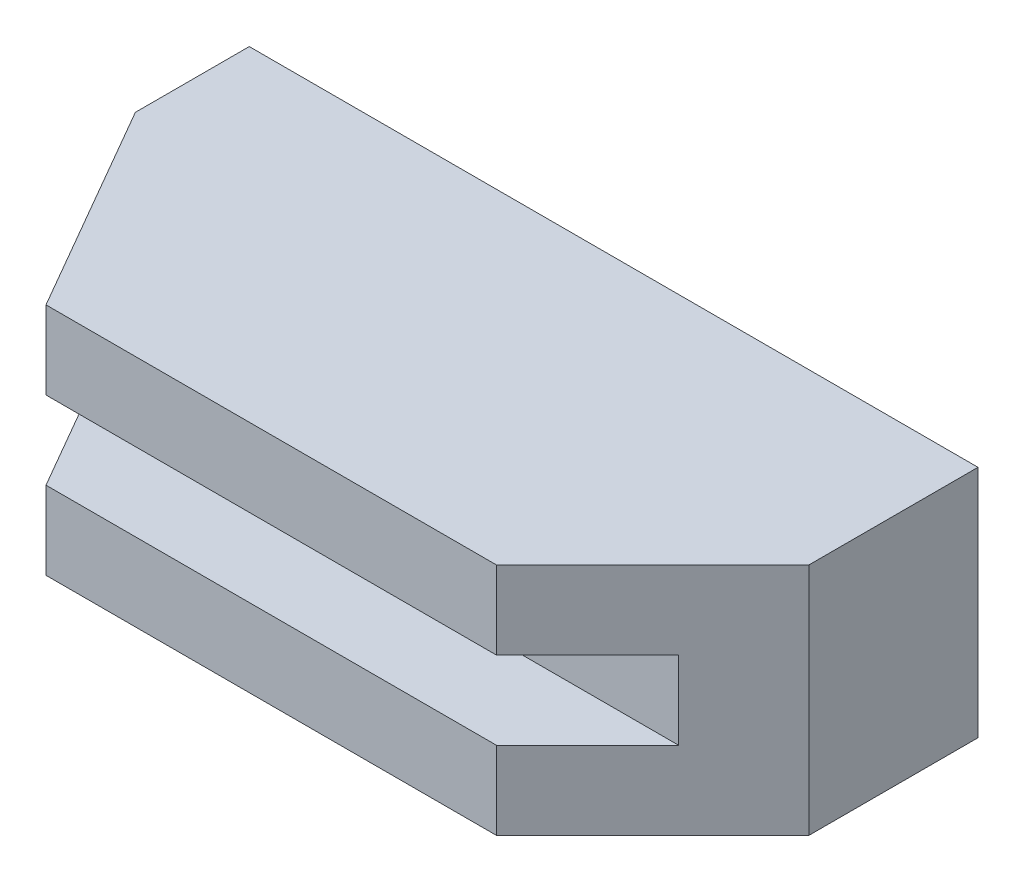
ISO-10303-21;
HEADER;
FILE_DESCRIPTION(('STEP AP214'),'2;1');
FILE_NAME('part.step','',(''),(''),'','','');
FILE_SCHEMA(('AUTOMOTIVE_DESIGN { 1 0 10303 214 1 1 1 1 }'));
ENDSEC;
DATA;
#1=APPLICATION_CONTEXT('core data for automotive mechanical design processes');
#2=APPLICATION_PROTOCOL_DEFINITION('international standard','automotive_design',2000,#1);
#3=PRODUCT_CONTEXT('',#1,'mechanical');
#4=PRODUCT('Part','Part','',(#3));
#5=PRODUCT_RELATED_PRODUCT_CATEGORY('part','',(#4));
#6=PRODUCT_DEFINITION_FORMATION('','',#4);
#7=PRODUCT_DEFINITION_CONTEXT('part definition',#1,'design');
#8=PRODUCT_DEFINITION('design','',#6,#7);
#9=PRODUCT_DEFINITION_SHAPE('','',#8);
#10=(LENGTH_UNIT() NAMED_UNIT(*) SI_UNIT(.MILLI.,.METRE.));
#11=(NAMED_UNIT(*) PLANE_ANGLE_UNIT() SI_UNIT($,.RADIAN.));
#12=(NAMED_UNIT(*) SI_UNIT($,.STERADIAN.) SOLID_ANGLE_UNIT());
#13=UNCERTAINTY_MEASURE_WITH_UNIT(LENGTH_MEASURE(1.E-05),#10,'distance_accuracy_value','');
#14=(GEOMETRIC_REPRESENTATION_CONTEXT(3) GLOBAL_UNCERTAINTY_ASSIGNED_CONTEXT((#13)) GLOBAL_UNIT_ASSIGNED_CONTEXT((#10,
#11,#12)) REPRESENTATION_CONTEXT('',''));
#15=CARTESIAN_POINT('',(0.,0.,0.));
#16=DIRECTION('',(0.,0.,1.));
#17=DIRECTION('',(1.,0.,0.));
#18=AXIS2_PLACEMENT_3D('',#15,#16,#17);
#19=CARTESIAN_POINT('',(0.,0.,25.));
#20=DIRECTION('',(0.,0.,-1.));
#21=DIRECTION('',(-1.,0.,0.));
#22=AXIS2_PLACEMENT_3D('',#19,#20,#21);
#23=PLANE('',#22);
#24=DIRECTION('',(0.,-1.,0.));
#25=VECTOR('',#24,1.);
#26=CARTESIAN_POINT('',(16.0000000000001,9.,25.));
#27=LINE('',#26,#25);
#28=CARTESIAN_POINT('',(16.0000000000001,-3.,25.));
#29=VERTEX_POINT('',#28);
#30=CARTESIAN_POINT('',(16.0000000000001,-9.,25.));
#31=VERTEX_POINT('',#30);
#32=EDGE_CURVE('E142',#29,#31,#27,.T.);
#33=ORIENTED_EDGE('',*,*,#32,.F.);
#34=DIRECTION('',(1.,0.,0.));
#35=VECTOR('',#34,1.);
#36=CARTESIAN_POINT('',(-23.5,-3.,25.));
#37=LINE('',#36,#35);
#38=CARTESIAN_POINT('',(-18.61984811475,-3.,25.));
#39=VERTEX_POINT('',#38);
#40=EDGE_CURVE('E136',#39,#29,#37,.T.);
#41=ORIENTED_EDGE('',*,*,#40,.F.);
#42=DIRECTION('',(0.,-1.,0.));
#43=VECTOR('',#42,1.);
#44=CARTESIAN_POINT('',(-18.61984811475,9.,25.));
#45=LINE('',#44,#43);
#46=CARTESIAN_POINT('',(-18.61984811475,-9.,25.));
#47=VERTEX_POINT('',#46);
#48=EDGE_CURVE('E65',#39,#47,#45,.T.);
#49=ORIENTED_EDGE('',*,*,#48,.T.);
#50=DIRECTION('',(1.,0.,0.));
#51=VECTOR('',#50,1.);
#52=CARTESIAN_POINT('',(-28.,-9.,25.));
#53=LINE('',#52,#51);
#54=EDGE_CURVE('E161',#47,#31,#53,.T.);
#55=ORIENTED_EDGE('',*,*,#54,.T.);
#56=EDGE_LOOP('',(#33,#41,#49,#55));
#57=FACE_BOUND('',#56,.T.);
#58=ADVANCED_FACE('F39',(#57),#23,.F.);
#59=CARTESIAN_POINT('',(28.,-9.,25.));
#60=DIRECTION('',(-1.,0.,0.));
#61=DIRECTION('',(0.,0.,1.));
#62=AXIS2_PLACEMENT_3D('',#59,#60,#61);
#63=PLANE('',#62);
#64=DIRECTION('',(0.,0.,-1.));
#65=VECTOR('',#64,1.);
#66=CARTESIAN_POINT('',(28.,9.,25.));
#67=LINE('',#66,#65);
#68=CARTESIAN_POINT('',(28.,9.,13.));
#69=VERTEX_POINT('',#68);
#70=CARTESIAN_POINT('',(28.,9.,0.));
#71=VERTEX_POINT('',#70);
#72=EDGE_CURVE('E180',#69,#71,#67,.T.);
#73=ORIENTED_EDGE('',*,*,#72,.F.);
#74=DIRECTION('',(0.,-1.,0.));
#75=VECTOR('',#74,1.);
#76=CARTESIAN_POINT('',(28.,9.,13.));
#77=LINE('',#76,#75);
#78=CARTESIAN_POINT('',(28.,-9.,13.));
#79=VERTEX_POINT('',#78);
#80=EDGE_CURVE('E143',#69,#79,#77,.T.);
#81=ORIENTED_EDGE('',*,*,#80,.T.);
#82=DIRECTION('',(0.,0.,-1.));
#83=VECTOR('',#82,1.);
#84=CARTESIAN_POINT('',(28.,-9.,25.));
#85=LINE('',#84,#83);
#86=CARTESIAN_POINT('',(28.,-9.,0.));
#87=VERTEX_POINT('',#86);
#88=EDGE_CURVE('E163',#79,#87,#85,.T.);
#89=ORIENTED_EDGE('',*,*,#88,.T.);
#90=DIRECTION('',(0.,1.,0.));
#91=VECTOR('',#90,1.);
#92=CARTESIAN_POINT('',(28.,-9.,0.));
#93=LINE('',#92,#91);
#94=EDGE_CURVE('E144',#87,#71,#93,.T.);
#95=ORIENTED_EDGE('',*,*,#94,.T.);
#96=EDGE_LOOP('',(#73,#81,#89,#95));
#97=FACE_BOUND('',#96,.T.);
#98=ADVANCED_FACE('F41',(#97),#63,.F.);
#99=CARTESIAN_POINT('',(-28.,9.,25.));
#100=DIRECTION('',(0.,-1.,0.));
#101=DIRECTION('',(0.,0.,-1.));
#102=AXIS2_PLACEMENT_3D('',#99,#100,#101);
#103=PLANE('',#102);
#104=DIRECTION('',(-1.,0.,0.));
#105=VECTOR('',#104,1.);
#106=CARTESIAN_POINT('',(-28.,9.,25.));
#107=LINE('',#106,#105);
#108=CARTESIAN_POINT('',(16.0000000000001,9.,25.));
#109=VERTEX_POINT('',#108);
#110=CARTESIAN_POINT('',(-18.61984811475,9.,25.));
#111=VERTEX_POINT('',#110);
#112=EDGE_CURVE('E157',#109,#111,#107,.T.);
#113=ORIENTED_EDGE('',*,*,#112,.F.);
#114=DIRECTION('',(0.707106781186544,0.,-0.707106781186551));
#115=VECTOR('',#114,1.);
#116=CARTESIAN_POINT('',(28.,9.,13.));
#117=LINE('',#116,#115);
#118=EDGE_CURVE('E140',#109,#69,#117,.T.);
#119=ORIENTED_EDGE('',*,*,#118,.T.);
#120=ORIENTED_EDGE('',*,*,#72,.T.);
#121=DIRECTION('',(-1.,0.,0.));
#122=VECTOR('',#121,1.);
#123=CARTESIAN_POINT('',(-28.,9.,0.));
#124=LINE('',#123,#122);
#125=CARTESIAN_POINT('',(-28.,9.,0.));
#126=VERTEX_POINT('',#125);
#127=EDGE_CURVE('E170',#71,#126,#124,.T.);
#128=ORIENTED_EDGE('',*,*,#127,.T.);
#129=DIRECTION('',(0.,0.,-1.));
#130=VECTOR('',#129,1.);
#131=CARTESIAN_POINT('',(-28.,9.,25.));
#132=LINE('',#131,#130);
#133=CARTESIAN_POINT('',(-28.,9.,8.75310035203402));
#134=VERTEX_POINT('',#133);
#135=EDGE_CURVE('E179',#134,#126,#132,.T.);
#136=ORIENTED_EDGE('',*,*,#135,.F.);
#137=DIRECTION('',(0.500000000000001,0.,0.866025403784438));
#138=VECTOR('',#137,1.);
#139=CARTESIAN_POINT('',(-28.,9.,8.75310035203402));
#140=LINE('',#139,#138);
#141=EDGE_CURVE('E149',#134,#111,#140,.T.);
#142=ORIENTED_EDGE('',*,*,#141,.T.);
#143=EDGE_LOOP('',(#113,#119,#120,#128,#136,#142));
#144=FACE_BOUND('',#143,.T.);
#145=ADVANCED_FACE('F212',(#144),#103,.F.);
#146=CARTESIAN_POINT('',(-28.,-9.,25.));
#147=DIRECTION('',(1.,0.,0.));
#148=DIRECTION('',(0.,0.,-1.));
#149=AXIS2_PLACEMENT_3D('',#146,#147,#148);
#150=PLANE('',#149);
#151=DIRECTION('',(0.,0.,-1.));
#152=VECTOR('',#151,1.);
#153=CARTESIAN_POINT('',(-28.,-9.,25.));
#154=LINE('',#153,#152);
#155=CARTESIAN_POINT('',(-28.,-9.,8.75310035203402));
#156=VERTEX_POINT('',#155);
#157=CARTESIAN_POINT('',(-28.,-9.,0.));
#158=VERTEX_POINT('',#157);
#159=EDGE_CURVE('E176',#156,#158,#154,.T.);
#160=ORIENTED_EDGE('',*,*,#159,.F.);
#161=DIRECTION('',(0.,-1.,0.));
#162=VECTOR('',#161,1.);
#163=CARTESIAN_POINT('',(-28.,9.,8.75310035203402));
#164=LINE('',#163,#162);
#165=EDGE_CURVE('E155',#134,#156,#164,.T.);
#166=ORIENTED_EDGE('',*,*,#165,.F.);
#167=ORIENTED_EDGE('',*,*,#135,.T.);
#168=DIRECTION('',(0.,-1.,0.));
#169=VECTOR('',#168,1.);
#170=CARTESIAN_POINT('',(-28.,-9.,0.));
#171=LINE('',#170,#169);
#172=EDGE_CURVE('E168',#126,#158,#171,.T.);
#173=ORIENTED_EDGE('',*,*,#172,.T.);
#174=EDGE_LOOP('',(#160,#166,#167,#173));
#175=FACE_BOUND('',#174,.T.);
#176=ADVANCED_FACE('F220',(#175),#150,.F.);
#177=CARTESIAN_POINT('',(-28.,-9.,25.));
#178=DIRECTION('',(0.,1.,0.));
#179=DIRECTION('',(0.,0.,1.));
#180=AXIS2_PLACEMENT_3D('',#177,#178,#179);
#181=PLANE('',#180);
#182=ORIENTED_EDGE('',*,*,#88,.F.);
#183=DIRECTION('',(0.707106781186544,0.,-0.707106781186551));
#184=VECTOR('',#183,1.);
#185=CARTESIAN_POINT('',(28.,-9.,13.));
#186=LINE('',#185,#184);
#187=EDGE_CURVE('E160',#31,#79,#186,.T.);
#188=ORIENTED_EDGE('',*,*,#187,.F.);
#189=ORIENTED_EDGE('',*,*,#54,.F.);
#190=DIRECTION('',(0.500000000000001,0.,0.866025403784438));
#191=VECTOR('',#190,1.);
#192=CARTESIAN_POINT('',(-28.,-9.,8.75310035203402));
#193=LINE('',#192,#191);
#194=EDGE_CURVE('E153',#156,#47,#193,.T.);
#195=ORIENTED_EDGE('',*,*,#194,.F.);
#196=ORIENTED_EDGE('',*,*,#159,.T.);
#197=DIRECTION('',(1.,0.,0.));
#198=VECTOR('',#197,1.);
#199=CARTESIAN_POINT('',(-28.,-9.,0.));
#200=LINE('',#199,#198);
#201=EDGE_CURVE('E165',#158,#87,#200,.T.);
#202=ORIENTED_EDGE('',*,*,#201,.T.);
#203=EDGE_LOOP('',(#182,#188,#189,#195,#196,#202));
#204=FACE_BOUND('',#203,.T.);
#205=ADVANCED_FACE('F201',(#204),#181,.F.);
#206=CARTESIAN_POINT('',(-18.61984811475,3.,25.));
#207=VERTEX_POINT('',#206);
#208=EDGE_CURVE('E134',#111,#207,#45,.T.);
#209=ORIENTED_EDGE('',*,*,#208,.T.);
#210=DIRECTION('',(-1.,0.,0.));
#211=VECTOR('',#210,1.);
#212=CARTESIAN_POINT('',(-23.5,3.,25.));
#213=LINE('',#212,#211);
#214=CARTESIAN_POINT('',(16.0000000000001,3.,25.));
#215=VERTEX_POINT('',#214);
#216=EDGE_CURVE('E119',#215,#207,#213,.T.);
#217=ORIENTED_EDGE('',*,*,#216,.F.);
#218=EDGE_CURVE('E132',#109,#215,#27,.T.);
#219=ORIENTED_EDGE('',*,*,#218,.F.);
#220=ORIENTED_EDGE('',*,*,#112,.T.);
#221=EDGE_LOOP('',(#209,#217,#219,#220));
#222=FACE_BOUND('',#221,.T.);
#223=ADVANCED_FACE('F131',(#222),#23,.F.);
#224=CARTESIAN_POINT('',(0.,0.,0.));
#225=DIRECTION('',(0.,0.,-1.));
#226=DIRECTION('',(-1.,0.,0.));
#227=AXIS2_PLACEMENT_3D('',#224,#225,#226);
#228=PLANE('',#227);
#229=ORIENTED_EDGE('',*,*,#94,.F.);
#230=ORIENTED_EDGE('',*,*,#201,.F.);
#231=ORIENTED_EDGE('',*,*,#172,.F.);
#232=ORIENTED_EDGE('',*,*,#127,.F.);
#233=EDGE_LOOP('',(#229,#230,#231,#232));
#234=FACE_BOUND('',#233,.T.);
#235=ADVANCED_FACE('F211',(#234),#228,.T.);
#236=CARTESIAN_POINT('',(-28.,9.,8.75310035203402));
#237=DIRECTION('',(0.866025403784438,0.,-0.500000000000001));
#238=DIRECTION('',(-0.500000000000001,0.,-0.866025403784438));
#239=AXIS2_PLACEMENT_3D('',#236,#237,#238);
#240=PLANE('',#239);
#241=ORIENTED_EDGE('',*,*,#48,.F.);
#242=DIRECTION('',(-0.500000000000001,0.,-0.866025403784438));
#243=VECTOR('',#242,1.);
#244=CARTESIAN_POINT('',(-28.,-3.,8.75310035203402));
#245=LINE('',#244,#243);
#246=CARTESIAN_POINT('',(-22.6612999990774,-3.,18.));
#247=VERTEX_POINT('',#246);
#248=EDGE_CURVE('E154',#39,#247,#245,.T.);
#249=ORIENTED_EDGE('',*,*,#248,.T.);
#250=DIRECTION('',(0.,1.,0.));
#251=VECTOR('',#250,1.);
#252=CARTESIAN_POINT('',(-22.6612999990774,9.,18.));
#253=LINE('',#252,#251);
#254=CARTESIAN_POINT('',(-22.6612999990774,3.,18.));
#255=VERTEX_POINT('',#254);
#256=EDGE_CURVE('E183',#247,#255,#253,.T.);
#257=ORIENTED_EDGE('',*,*,#256,.T.);
#258=DIRECTION('',(0.500000000000001,0.,0.866025403784438));
#259=VECTOR('',#258,1.);
#260=CARTESIAN_POINT('',(-28.,3.,8.75310035203402));
#261=LINE('',#260,#259);
#262=EDGE_CURVE('E189',#255,#207,#261,.T.);
#263=ORIENTED_EDGE('',*,*,#262,.T.);
#264=ORIENTED_EDGE('',*,*,#208,.F.);
#265=ORIENTED_EDGE('',*,*,#141,.F.);
#266=ORIENTED_EDGE('',*,*,#165,.T.);
#267=ORIENTED_EDGE('',*,*,#194,.T.);
#268=EDGE_LOOP('',(#241,#249,#257,#263,#264,#265,#266,#267));
#269=FACE_BOUND('',#268,.T.);
#270=ADVANCED_FACE('F188',(#269),#240,.F.);
#271=CARTESIAN_POINT('',(28.,9.,13.));
#272=DIRECTION('',(-0.707106781186551,0.,-0.707106781186544));
#273=DIRECTION('',(-0.707106781186544,0.,0.707106781186551));
#274=AXIS2_PLACEMENT_3D('',#271,#272,#273);
#275=PLANE('',#274);
#276=DIRECTION('',(0.,-1.,0.));
#277=VECTOR('',#276,1.);
#278=CARTESIAN_POINT('',(23.0000000000001,9.,18.));
#279=LINE('',#278,#277);
#280=CARTESIAN_POINT('',(23.0000000000001,3.,18.));
#281=VERTEX_POINT('',#280);
#282=CARTESIAN_POINT('',(23.0000000000001,-3.,18.));
#283=VERTEX_POINT('',#282);
#284=EDGE_CURVE('E130',#281,#283,#279,.T.);
#285=ORIENTED_EDGE('',*,*,#284,.T.);
#286=DIRECTION('',(-0.707106781186544,0.,0.707106781186551));
#287=VECTOR('',#286,1.);
#288=CARTESIAN_POINT('',(28.,-3.,13.));
#289=LINE('',#288,#287);
#290=EDGE_CURVE('E11',#283,#29,#289,.T.);
#291=ORIENTED_EDGE('',*,*,#290,.T.);
#292=ORIENTED_EDGE('',*,*,#32,.T.);
#293=ORIENTED_EDGE('',*,*,#187,.T.);
#294=ORIENTED_EDGE('',*,*,#80,.F.);
#295=ORIENTED_EDGE('',*,*,#118,.F.);
#296=ORIENTED_EDGE('',*,*,#218,.T.);
#297=DIRECTION('',(0.707106781186544,0.,-0.707106781186551));
#298=VECTOR('',#297,1.);
#299=CARTESIAN_POINT('',(28.,3.,13.));
#300=LINE('',#299,#298);
#301=EDGE_CURVE('E50',#215,#281,#300,.T.);
#302=ORIENTED_EDGE('',*,*,#301,.T.);
#303=EDGE_LOOP('',(#285,#291,#292,#293,#294,#295,#296,#302));
#304=FACE_BOUND('',#303,.T.);
#305=ADVANCED_FACE('F139',(#304),#275,.F.);
#306=CARTESIAN_POINT('',(-23.5,-3.,18.));
#307=DIRECTION('',(0.,-1.,0.));
#308=DIRECTION('',(0.,0.,-1.));
#309=AXIS2_PLACEMENT_3D('',#306,#307,#308);
#310=PLANE('',#309);
#311=ORIENTED_EDGE('',*,*,#40,.T.);
#312=ORIENTED_EDGE('',*,*,#290,.F.);
#313=DIRECTION('',(1.,0.,0.));
#314=VECTOR('',#313,1.);
#315=CARTESIAN_POINT('',(-23.5,-3.,18.));
#316=LINE('',#315,#314);
#317=EDGE_CURVE('E53',#247,#283,#316,.T.);
#318=ORIENTED_EDGE('',*,*,#317,.F.);
#319=ORIENTED_EDGE('',*,*,#248,.F.);
#320=EDGE_LOOP('',(#311,#312,#318,#319));
#321=FACE_BOUND('',#320,.T.);
#322=ADVANCED_FACE('F245',(#321),#310,.F.);
#323=CARTESIAN_POINT('',(-23.5,3.,18.));
#324=DIRECTION('',(0.,1.,0.));
#325=DIRECTION('',(0.,0.,1.));
#326=AXIS2_PLACEMENT_3D('',#323,#324,#325);
#327=PLANE('',#326);
#328=DIRECTION('',(-1.,0.,0.));
#329=VECTOR('',#328,1.);
#330=CARTESIAN_POINT('',(-23.5,3.,18.));
#331=LINE('',#330,#329);
#332=EDGE_CURVE('E124',#281,#255,#331,.T.);
#333=ORIENTED_EDGE('',*,*,#332,.F.);
#334=ORIENTED_EDGE('',*,*,#301,.F.);
#335=ORIENTED_EDGE('',*,*,#216,.T.);
#336=ORIENTED_EDGE('',*,*,#262,.F.);
#337=EDGE_LOOP('',(#333,#334,#335,#336));
#338=FACE_BOUND('',#337,.T.);
#339=ADVANCED_FACE('F118',(#338),#327,.F.);
#340=CARTESIAN_POINT('',(0.,0.,18.));
#341=DIRECTION('',(0.,0.,-1.));
#342=DIRECTION('',(-1.,0.,0.));
#343=AXIS2_PLACEMENT_3D('',#340,#341,#342);
#344=PLANE('',#343);
#345=ORIENTED_EDGE('',*,*,#317,.T.);
#346=ORIENTED_EDGE('',*,*,#284,.F.);
#347=ORIENTED_EDGE('',*,*,#332,.T.);
#348=ORIENTED_EDGE('',*,*,#256,.F.);
#349=EDGE_LOOP('',(#345,#346,#347,#348));
#350=FACE_BOUND('',#349,.T.);
#351=ADVANCED_FACE('F181',(#350),#344,.F.);
#352=CLOSED_SHELL('',(#58,#98,#145,#176,#205,#223,#235,#270,#305,#322,#339,#351));
#353=MANIFOLD_SOLID_BREP('B2',#352);
#354=ADVANCED_BREP_SHAPE_REPRESENTATION('',(#18,#353),#14);
#355=SHAPE_DEFINITION_REPRESENTATION(#9,#354);
ENDSEC;
END-ISO-10303-21;
